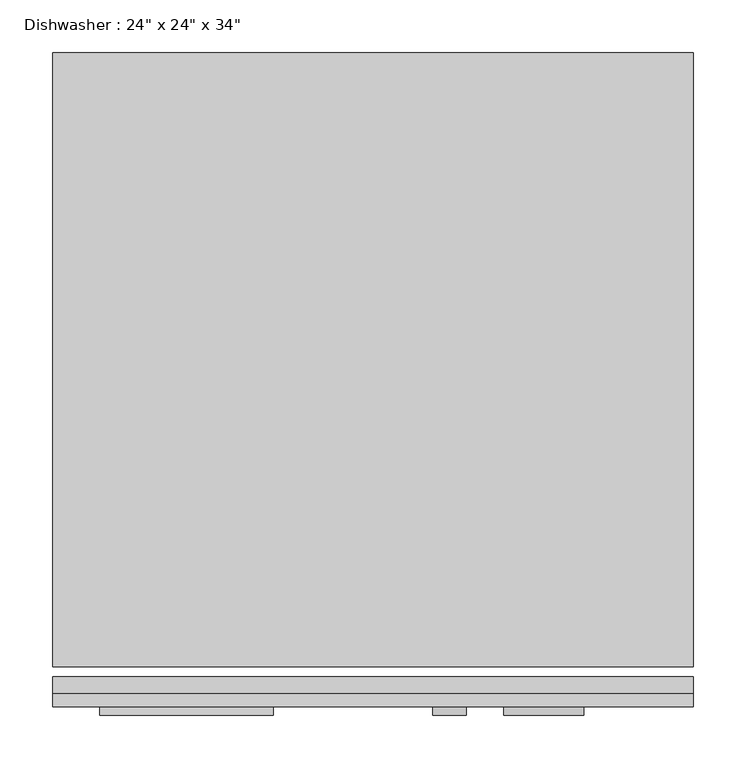
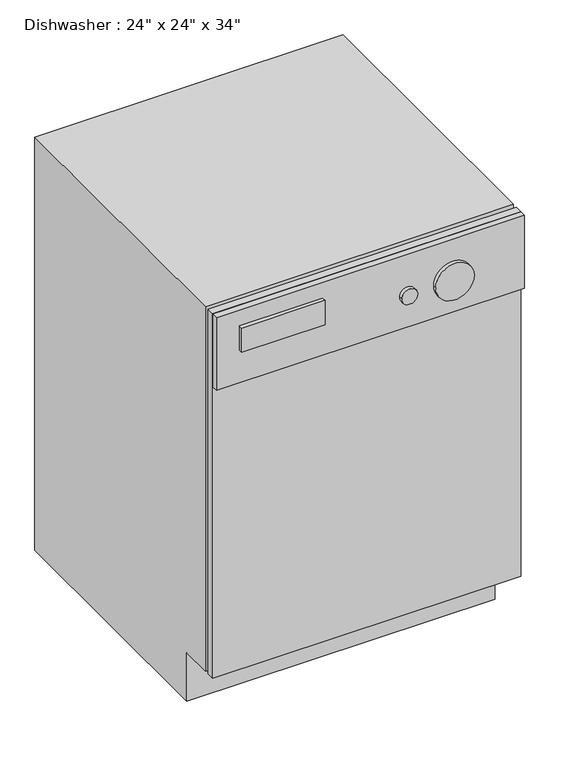
"""IFC4 building model written with IfcOpenShell, lengths in millimetres: proxy geometry."""

from ifc_helpers import new_model, si_unit, point, frame, frame_2d, origin, place, context, project, spatial, polyline, circle_curve, trimmed, segment, composite_curve, outline, extrude, source, transform, mapped, element, save


def proxy_45b28599(model_context):
    return source(origin(), model_context, "Body", "SweptSolid", [
        extrude(outline(polyline([(687.1174685, -38.3504352), (77.5174685, -38.3504352), (77.5174685, -22.4754352), (687.1174685, -22.4754352), (687.1174685, -38.3504352)])), frame((0.0, 0.0, 101.6), z_axis=(0.0, 0.0, 1.0), x_axis=(1.0, 0.0, 0.0)), (0.0, 0.0, 1.0), 762.0),
        extrude(outline(polyline([(687.1174685, -38.3504352), (687.1174685, -51.0504352), (77.5174685, -51.0504352), (77.5174685, -38.3504352), (687.1174685, -38.3504352)])), frame((0.0, 0.0, 711.2), z_axis=(0.0, 0.0, 1.0), x_axis=(1.0, 0.0, 0.0)), (0.0, 0.0, 1.0), 152.4),
        extrude(outline(polyline([(571.2495648, 0.0), (50.5495648, 0.0), (50.5495648, 101.6), (-12.9504352, 101.6), (-12.9504352, 863.6), (571.2495648, 863.6), (571.2495648, 0.0)])), frame((77.5174685, 0.0, 0.0), z_axis=(1.0, 0.0, 0.0), x_axis=(0.0, 1.0, 0.0)), (0.0, 0.0, 1.0), 609.6),
        extrude(outline(polyline([(287.6378068, -59.1863727), (122.5378068, -59.1863727), (122.5378068, -51.0504352), (287.6378068, -51.0504352), (287.6378068, -59.1863727)])), frame((0.0, 0.0, 780.0846419), z_axis=(0.0, 0.0, 1.0), x_axis=(1.0, 0.0, 0.0)), (0.0, 0.0, 1.0), 50.8),
        extrude(outline(composite_curve([segment(trimmed(circle_curve(frame_2d((780.0846419, 544.7247133)), 38.1), [point((780.0846419, 506.6247133))], [point((780.0846419, 582.8247133))], False, "CARTESIAN"), True, "CONTINUOUS"), segment(trimmed(circle_curve(frame_2d((780.0846419, 544.7247133)), 38.1), [point((780.0846419, 582.8247133))], [point((780.0846419, 506.6247133))], False, "CARTESIAN"), True, "CONTINUOUS")], self_intersect=False)), frame((0.0, -59.1863727, 0.0), z_axis=(0.0, 1.0, 0.0), x_axis=(0.0, 0.0, 1.0)), (0.0, 0.0, 1.0), 8.1359375),
        extrude(outline(composite_curve([segment(trimmed(circle_curve(frame_2d((780.0846419, 455.195318)), 15.875), [point((780.0846419, 439.320318))], [point((780.0846419, 471.070318))], False, "CARTESIAN"), True, "CONTINUOUS"), segment(trimmed(circle_curve(frame_2d((780.0846419, 455.195318)), 15.875), [point((780.0846419, 471.070318))], [point((780.0846419, 439.320318))], False, "CARTESIAN"), True, "CONTINUOUS")], self_intersect=False)), frame((0.0, -59.1863727, 0.0), z_axis=(0.0, 1.0, 0.0), x_axis=(0.0, 0.0, 1.0)), (0.0, 0.0, 1.0), 8.1359375),
    ])


if __name__ == "__main__":
    model = new_model("IFC4")
    model_context = context("Model", 3, world=origin())
    ifc_project = project(units=[si_unit("LENGTHUNIT", "METRE", prefix="MILLI")], contexts=[model_context])
    site = spatial("IfcSite", under=ifc_project)
    building = spatial("IfcBuilding", under=site)
    placement = place(None, origin())
    proxy_shape = proxy_45b28599(model_context)
    element("IfcBuildingElementProxy", 1, Name="Dishwasher : 24\" x 24\" x 34\"", ObjectType="Dishwasher : 24\" x 24\" x 34\"", at=placement, inside=building, context=model_context, shape_type="MappedRepresentation", body=[
        mapped(proxy_shape, transform((0.0, 0.0, 0.0), x_axis=(1.0, 0.0, 0.0), y_axis=(0.0, 1.0, 0.0), z_axis=(0.0, 0.0, 1.0))),
    ])
    save(model, "model.ifc")

# Revit data of these elements
# Type "Dishwasher : 24\" x 24\" x 34\""
#   Label = "DW"
#   Assembly Code = "E1090400"
#   Depth = 2' - 0"
#   Height = 2' - 10"
#   Width = 2' - 0"
#   Dishwasher Material = Steel, Paint Finish, Ivory, Glossy
#   Panel Face Material = Plastic, Opaque Black
#   Default Elevation = 0
# Element 1 (IfcBuildingElementProxy, "Dishwasher : 24\" x 24\" x 34\"")
#   Materials on its faces: "Steel, Paint Finish, Ivory, Glossy", "Plastic, Opaque Black"
# Materials
#   "Steel, Paint Finish, Ivory, Glossy": class "Metal", colour RGB 247 247 239, transparency 0, Description = "Steel, paint finish, ivory, glossy", Cost = 0
#   "Plastic, Opaque Black": class "Plastic", colour RGB 0 0 0, transparency 0, Description = "Plastic, generic, opaque black", Cost = 0
